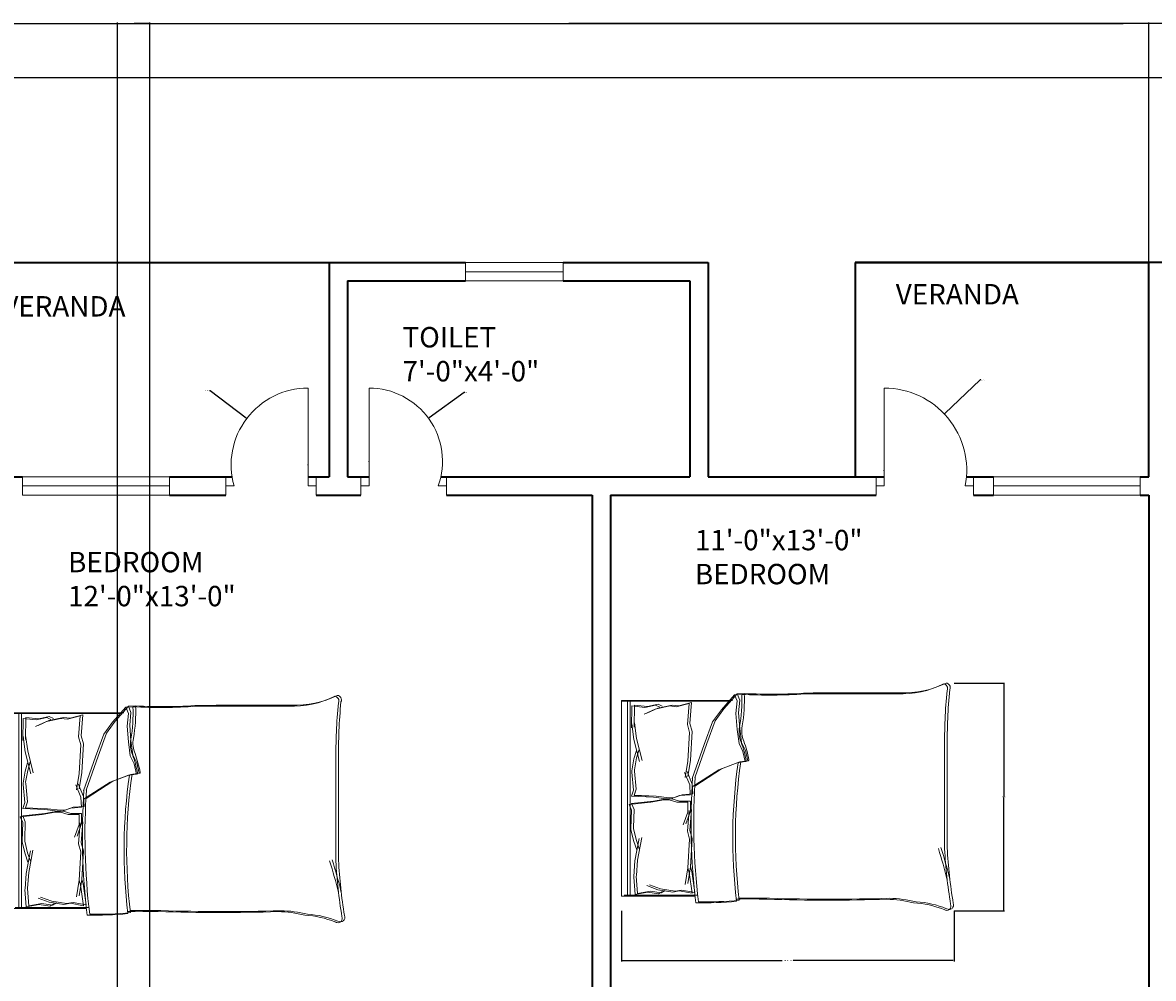
# Model space of a CAD drawing. Units: inches. Extents: x 2163 to 2982, y 1024 to 2288.
# Tile 18 of 22: x 2306 to 2583, y 2054 to 2288. Entities that reach past the tile are written whole.
import ezdxf

# ---------------------------------------------------------------- set-up
doc = ezdxf.new("R2010")
doc.units = ezdxf.units.IN
for name, color, linetype, lineweight in [('A-ANNO-DIMS', 2, 'Continuous', 18), ('A-ANNO-TTLB', 7, 'Continuous', 25), ('A-AREA-IDEN', 7, 'Continuous', 18), ('A-DOOR', 11, 'Continuous', 18), ('A-FURN', 8, 'Continuous', 13), ('A-GLAZ', 161, 'Continuous', 18), ('A-WALL', 7, 'Continuous', 35)]:
    doc.layers.add(name, color=color, linetype=linetype, lineweight=lineweight)
doc.styles.get("Standard").update_dxf_attribs({"font": 'arial.ttf'})
doc.dimstyles.get("Standard").update_dxf_attribs({"dimtxt": 0.18, "dimasz": 0.18, "dimexe": 0.18, "dimexo": 0.0625, "dimgap": 0.09, "dimtad": 0, "dimtih": 1, "dimtoh": 1, "dimdec": 4, "dimzin": 0, "dimdsep": 46, "dimtxsty": 'Standard', "dimcen": 0.09, "dimadec": 0, "dimazin": 0, "dimtfac": 1, "dimtdec": 4, "dimtofl": 0, "dimtmove": 0, "dimatfit": 3, "dimfxl": 1, "dimtolj": 1, "dimtzin": 0, "dimarcsym": 0})

# ---------------------------------------------------------------- blocks, each defined once
blk = doc.blocks.new('BED-DOUBLE')
for p, q in [((27.75, 52.87), (24.5, 49.16)), ((27.75, 52.87), (24.5, 49.16)), ((28.38, 53.1), (25.13, 49.39)), ((28.38, 53.1), (25.13, 49.39)), ((29.49, 52.95), (27.75, 52.87, 3.87)), ((29.49, 52.95), (27.75, 52.87, 3.87)), ((28.36, 51.33), (27.75, 52.87)), ((28.36, 51.33), (27.75, 52.87)), ((30.13, 53.18), (28.38, 53.1, 3.87)), ((29, 51.56), (28.38, 53.1)), ((30.13, 53.18), (28.38, 53.1, 3.87)), ((29, 51.56), (28.38, 53.1)), ((0, 51.49), (0.64, 51.49)), ((0, 3.47), (0, 51.49)), ((0, 51.27), (26.61, 51.27)), ((0, 51.27), (26.61, 51.27)), ((0.64, 51.49), (27.25, 51.49)), ((0.64, 51.49), (27.25, 51.49)), ((1.53, 3.48), (1.53, 51.27)), ((1.53, 3.47), (1.53, 51.27)), ((2.17, 3.7), (2.17, 51.49)), ((2.17, 3.7), (2.17, 51.49)), ((2.56, 50.11), (2.46, 44.71)), ((2.56, 50.11), (2.46, 44.71)), ((2.56, 50.11), (5.77, 49.73)), ((2.56, 50.11), (5.77, 49.73)), ((3.2, 50.34), (3.1, 44.94)), ((3.2, 50.34), (3.1, 44.94)), ((3.2, 50.34), (6.41, 49.96)), ((3.2, 50.34), (6.41, 49.96)), ((5.77, 49.73), (8.34, 50.33)), ((5.77, 49.73), (8.34, 50.33)), ((6.41, 49.96), (8.98, 50.56)), ((6.41, 49.96), (8.98, 50.56)), ((11.83, 50.11), (8.26, 49.31)), ((11.83, 50.11), (8.26, 49.31)), ((8.34, 50.33), (9.38, 49.81)), ((8.34, 50.33), (9.38, 49.81)), ((12.47, 50.34), (8.9, 49.54)), ((12.47, 50.34), (8.9, 49.54)), ((8.98, 50.56), (10.02, 50.04)), ((8.98, 50.56), (10.02, 50.04)), ((13.43, 49.92), (11.83, 50.11)), ((13.43, 49.92), (11.83, 50.11)), ((14.07, 50.15), (12.47, 50.34)), ((14.07, 50.15), (12.47, 50.34)), ((16.57, 50.7), (13.43, 49.92)), ((16.57, 50.7), (13.43, 49.92)), ((17.21, 50.93), (14.07, 50.15)), ((17.21, 50.93), (14.07, 50.15)), ((16.17, 45.57), (16.57, 50.7)), ((16.17, 45.57), (16.57, 50.7)), ((16.81, 45.79), (17.21, 50.93)), ((16.81, 45.79), (17.21, 50.93)), ((28.06, 48.23), (28.36, 51.33)), ((28.06, 48.23), (28.36, 51.33)), ((28.69, 48.46), (29, 51.56)), ((28.69, 48.46), (29, 51.56)), ((8.26, 49.31), (5.58, 48.13)), ((8.26, 49.31), (5.58, 48.13)), ((8.9, 49.54), (6.22, 48.36)), ((8.9, 49.54), (6.22, 48.36)), ((24.5, 49.16), (22.33, 46.22)), ((24.5, 49.16), (22.33, 46.22)), ((25.13, 49.39), (22.97, 46.45)), ((25.13, 49.39), (22.97, 46.45)), ((28.36, 44.36), (28.06, 48.23)), ((28.36, 44.36), (28.06, 48.23)), ((29, 44.59), (28.69, 48.46)), ((29, 44.59), (28.69, 48.46)), ((2.46, 44.71), (2.54, 45.71)), ((2.46, 44.71), (2.54, 45.71)), ((2.54, 45.71), (3.07, 41.91)), ((2.54, 45.71), (3.07, 41.91)), ((3.1, 44.94), (3.18, 45.94)), ((3.1, 44.94), (3.18, 45.94)), ((3.18, 45.94), (3.71, 42.14)), ((3.18, 45.94), (3.71, 42.14)), ((16.73, 43.61), (16.17, 45.57)), ((16.73, 43.61), (16.17, 45.57)), ((17.37, 43.83), (16.81, 45.79)), ((17.37, 43.83), (16.81, 45.79)), ((22.33, 46.22), (20.32, 40.64)), ((22.33, 46.22), (20.32, 40.64)), ((22.97, 46.45), (20.96, 40.87)), ((22.97, 46.45), (20.96, 40.87)), ((28.83, 40.95), (28.36, 44.36)), ((29.47, 41.18), (29, 44.59)), ((29.47, 41.18), (29, 44.59)), ((3.07, 41.91), (4.42, 36.49)), ((3.07, 41.91), (4.42, 36.49)), ((3.71, 42.14), (5.06, 36.72)), ((3.71, 42.14), (5.06, 36.72)), ((16.29, 36.6), (16.73, 43.61)), ((16.29, 36.6), (16.73, 43.61)), ((16.93, 36.82), (17.37, 43.83)), ((16.93, 36.82), (17.37, 43.83)), ((28.83, 40.95), (28.36, 44.36)), ((3.67, 39.2), (3.08, 37.14)), ((3.67, 39.2), (3.08, 37.13)), ((4.31, 39.43), (3.72, 37.36)), ((4.31, 39.43), (3.72, 37.36)), ((20.32, 40.64), (17.38, 32.31)), ((20.32, 40.64), (17.38, 32.31)), ((20.96, 40.87), (18.02, 32.53)), ((20.96, 40.87), (18.02, 32.53)), ((29.76, 38.94), (28.83, 40.95)), ((29.76, 38.94), (28.83, 40.95)), ((30.4, 39.17), (29.47, 41.18)), ((30.4, 39.17), (29.47, 41.18)), ((30.38, 36.46), (29.76, 38.94)), ((30.38, 36.46), (29.76, 38.94)), ((31.02, 36.69), (30.4, 39.17)), ((31.02, 36.69), (30.4, 39.17)), ((79.24, 15.06), (79.24, 39.68)), ((79.24, 15.06), (79.24, 39.68)), ((79.88, 15.29), (79.88, 39.91)), ((79.88, 15.29), (79.88, 39.91)), ((3.08, 37.14), (2.54, 34.2)), ((3.08, 37.13), (2.54, 34.2)), ((3.72, 37.36), (3.18, 34.43)), ((3.72, 37.36), (3.18, 34.43)), ((15.63, 32.56), (16.29, 36.6)), ((15.63, 32.56), (16.29, 36.6)), ((16.27, 32.79), (16.93, 36.82)), ((16.27, 32.79), (16.93, 36.82)), ((23.88, 34.45), (28.36, 36.15)), ((23.88, 34.45), (28.36, 36.15)), ((24.52, 34.68), (29, 36.38)), ((24.52, 34.68), (29, 36.38)), ((28.36, 36.15), (30.38, 36.46)), ((28.36, 36.15), (30.38, 36.46)), ((29, 36.38), (31.02, 36.69)), ((29, 36.38), (31.02, 36.69)), ((2.54, 34.2), (2.56, 33.88)), ((2.54, 34.2), (2.56, 33.88)), ((2.56, 33.88), (2.98, 29.46)), ((2.56, 33.88), (2.98, 29.46)), ((3.18, 34.43), (3.2, 34.11)), ((3.18, 34.43), (3.2, 34.11)), ((3.2, 34.11), (3.62, 29.68)), ((3.2, 34.11), (3.62, 29.68)), ((16.74, 30.75), (15.45, 33.82)), ((16.74, 30.75), (15.45, 33.82)), ((17.38, 30.98), (16.09, 34.05)), ((17.38, 30.98), (16.09, 34.05)), ((17.38, 30.26), (23.88, 34.45)), ((17.38, 30.26), (23.88, 34.45)), ((18.02, 30.49), (24.52, 34.68)), ((18.02, 30.49), (24.52, 34.68)), ((16.89, 28.3), (16.74, 30.75)), ((16.89, 28.3), (16.74, 30.75)), ((17.53, 28.53), (17.38, 30.98)), ((17.53, 28.53), (17.38, 30.98)), ((2.98, 29.46), (2.49, 27.98)), ((2.98, 29.46), (2.49, 27.98)), ((2.49, 27.98), (7.87, 27.73)), ((2.49, 27.98), (7.87, 27.73)), ((3.62, 29.68), (3.13, 28.21)), ((3.62, 29.68), (3.13, 28.2)), ((3.13, 28.21), (8.51, 27.96)), ((3.13, 28.2), (8.51, 27.96)), ((7.87, 27.73), (11.08, 27.35)), ((7.87, 27.73), (11.08, 27.35)), ((8.51, 27.96), (11.72, 27.58)), ((8.51, 27.96), (11.72, 27.58)), ((12.38, 27.44), (14.22, 28.13)), ((12.38, 27.44), (14.22, 28.13)), ((13.02, 27.66), (14.86, 28.36)), ((13.02, 27.66), (14.86, 28.36)), ((14.22, 28.13), (16.89, 28.3)), ((14.22, 28.13), (16.89, 28.3)), ((14.86, 28.36), (17.53, 28.53)), ((14.86, 28.36), (17.53, 28.53)), ((1.87, 25.98), (7.22, 26.56)), ((1.87, 25.98), (7.22, 26.56)), ((2.45, 24.54), (1.87, 25.98)), ((2.45, 24.54), (1.87, 25.98)), ((2.51, 26.21), (7.86, 26.79)), ((2.51, 26.21), (7.86, 26.79)), ((3.09, 24.77), (2.51, 26.21)), ((3.09, 24.77), (2.51, 26.21)), ((7.22, 26.56), (10.4, 27.14)), ((7.22, 26.56), (10.4, 27.14)), ((7.86, 26.79), (11.04, 27.37)), ((7.86, 26.79), (11.04, 27.37)), ((10.4, 27.14), (11.7, 27.14)), ((10.4, 27.14), (11.7, 27.14)), ((11.04, 27.37), (12.34, 27.37)), ((11.04, 27.37), (12.34, 27.37)), ((11.08, 27.35), (12.38, 27.44)), ((11.08, 27.35), (12.38, 27.44)), ((11.7, 27.14), (13.58, 26.56)), ((11.7, 27.14), (13.58, 26.56)), ((11.72, 27.58), (13.02, 27.66)), ((11.72, 27.58), (13.02, 27.66)), ((12.34, 27.37), (14.22, 26.79)), ((12.34, 27.37), (14.22, 26.79)), ((13.58, 26.56), (16.26, 26.56)), ((13.58, 26.56), (16.26, 26.56)), ((14.22, 26.79), (16.9, 26.79)), ((14.22, 26.79), (16.9, 26.79)), ((16.26, 26.56), (16.26, 24.1)), ((16.26, 26.56), (16.26, 24.1)), ((16.9, 26.79), (16.9, 24.33)), ((16.9, 26.79), (16.9, 24.33)), ((2.3, 20.09), (2.45, 24.54)), ((2.3, 20.09), (2.45, 24.54)), ((2.94, 20.32), (3.09, 24.77)), ((2.94, 20.32), (3.09, 24.77)), ((16.26, 24.1), (15.17, 20.96)), ((16.26, 24.1), (15.17, 20.96)), ((16.9, 24.33), (15.81, 21.19)), ((16.9, 24.33), (15.81, 21.19)), ((16.17, 19.38), (16.57, 24.52)), ((16.17, 19.38), (16.57, 24.52)), ((16.81, 19.61), (17.21, 24.74)), ((16.81, 19.61), (17.21, 24.74)), ((2.3, 19.77), (2.3, 20.09)), ((2.3, 19.77), (2.3, 20.09)), ((3.03, 16.88), (2.3, 19.77)), ((3.03, 16.88), (2.3, 19.77)), ((2.94, 20), (2.94, 20.32)), ((2.94, 20), (2.94, 20.32)), ((3.67, 17.11), (2.94, 20)), ((3.67, 17.11), (2.94, 20)), ((17.37, 17.65), (16.81, 19.61)), ((17.37, 17.65), (16.81, 19.61)), ((3.75, 14.85), (3.03, 16.88)), ((3.75, 14.85), (3.03, 16.88)), ((3.32, 12.11), (4.33, 17.6)), ((3.32, 12.11), (4.33, 17.6)), ((4.39, 15.08), (3.67, 17.11)), ((4.39, 15.08), (3.67, 17.11)), ((3.96, 12.34), (4.97, 17.83)), ((3.96, 12.34), (4.97, 17.83)), ((16.73, 17.42), (16.17, 19.38)), ((16.73, 17.42), (16.17, 19.38)), ((16.29, 10.41), (16.73, 17.42)), ((16.29, 10.41), (16.73, 17.42)), ((16.93, 10.64), (17.37, 17.65)), ((16.93, 10.64), (17.37, 17.65)), ((3.03, 8.28), (3.32, 12.11)), ((3.03, 8.28), (3.32, 12.11)), ((3.67, 8.51), (3.96, 12.34)), ((3.67, 8.51), (3.96, 12.34)), ((3.65, 8.41), (3.67, 8.51)), ((3.65, 8.41), (3.67, 8.51)), ((3.98, 4.13), (3.65, 8.41)), ((3.98, 4.13), (3.65, 8.41)), ((15.63, 6.38), (16.29, 10.41)), ((15.63, 6.38), (16.29, 10.41)), ((16.27, 6.61), (16.93, 10.64)), ((16.27, 6.61), (16.93, 10.64)), ((16.29, 10.41), (16.62, 9.28)), ((16.29, 10.41), (16.62, 9.28)), ((16.62, 9.28), (17.34, 4.18)), ((16.62, 9.28), (17.34, 4.18)), ((16.93, 10.64), (17.26, 9.51)), ((16.93, 10.64), (17.26, 9.51)), ((17.26, 9.51), (17.98, 4.41)), ((17.26, 9.51), (17.98, 4.41)), ((3.01, 8.18), (3.03, 8.28)), ((3.01, 8.18), (3.03, 8.28)), ((3.34, 3.9), (3.01, 8.18)), ((3.34, 3.9), (3.01, 8.18)), ((8.95, 5.05), (6.21, 6.06)), ((8.95, 5.05), (6.21, 6.06)), ((9.59, 5.28), (6.85, 6.29)), ((9.59, 5.28), (6.85, 6.29)), ((18.11, 3.48), (0, 3.48)), ((18.11, 3.47), (0, 3.47)), ((18.75, 3.7), (0.64, 3.7)), ((18.75, 3.7), (0.64, 3.7)), ((3.32, 3.89), (6.5, 4.47)), ((3.32, 3.89), (6.5, 4.47)), ((3.96, 4.12), (7.14, 4.7)), ((3.96, 4.12), (7.14, 4.7)), ((6.5, 4.47), (9.1, 4.04)), ((6.5, 4.47), (9.1, 4.04)), ((7.14, 4.7), (9.74, 4.27)), ((7.14, 4.7), (9.74, 4.27)), ((12.57, 4.47), (8.95, 5.05)), ((12.57, 4.47), (8.95, 5.05)), ((9.1, 4.04), (10.11, 4.62)), ((9.1, 4.04), (10.11, 4.62)), ((13.21, 4.7), (9.59, 5.28)), ((13.21, 4.7), (9.59, 5.28)), ((9.74, 4.27), (10.75, 4.85)), ((9.74, 4.27), (10.75, 4.85)), ((14.16, 4.76), (12.57, 4.47)), ((14.16, 4.76), (12.57, 4.47)), ((14.8, 4.99), (13.21, 4.7)), ((14.8, 4.99), (13.21, 4.7)), ((17.34, 4.18), (14.16, 4.76)), ((17.34, 4.18), (14.16, 4.76)), ((17.98, 4.41), (14.8, 4.99)), ((17.98, 4.41), (14.8, 4.99))]:
    blk.add_line(p, q)
for centre, radius, start, end in [((68.67, 76.16), 23.07, 267.4714, 296.4681), ((68.67, 76.16), 23.07, 267.4714, 296.4681), ((69.31, 76.39), 23.07, 267.4714, 296.4681), ((69.31, 76.39), 23.07, 267.4714, 296.4681), ((78.87, 54.41), 1.1, 332.6588, 86.02), ((78.87, 54.41), 1.1, 332.6588, 86.02), ((79.51, 54.64), 1.1, 332.6588, 86.02), ((79.51, 54.64), 1.1, 332.6588, 86.02), ((-6.66, 51.33), 36.18, 349.8763, 2.5657), ((-6.66, 51.33), 36.18, 349.8763, 2.5657), ((36.31, 182.27), 129.5, 266.9791, 273.8365), ((36.31, 182.27), 129.5, 266.9791, 273.8365), ((-6.02, 51.56), 36.18, 349.8763, 2.5657), ((-6.02, 51.56), 36.18, 349.8763, 2.5657), ((36.95, 182.49), 129.5, 266.9791, 273.8365), ((36.95, 182.49), 129.5, 266.9791, 273.8365), ((67.82, -4508.74), 4561.86, 90.00217, 90.28689), ((67.82, -4508.74), 4561.86, 90.00217, 90.28689), ((68.46, -4508.52), 4561.86, 90.00217, 90.28689), ((68.46, -4508.52), 4561.86, 90.00217, 90.28689), ((212.28, 41.15), 133.04, 174.4998, 180.6351), ((212.28, 41.15), 133.04, 174.4998, 180.6351), ((212.92, 41.38), 133.04, 174.4998, 180.6351), ((212.92, 41.38), 133.04, 174.4998, 180.6351), ((35.07, 43.74), 6.22, 168.6608, 203.7384), ((35.07, 43.74), 6.22, 168.6608, 203.7384), ((35.71, 43.97), 6.22, 168.6608, 203.7384), ((35.71, 43.97), 6.22, 168.6608, 203.7384), ((1.48, 31.15), 29.65, 10.6617, 19.8806), ((1.48, 31.15), 29.65, 10.6617, 19.8806), ((2.12, 31.38), 29.65, 10.6617, 19.8806), ((2.12, 31.38), 29.65, 10.6617, 19.8806), ((156.32, 17.76), 129.02, 171.7845, 186.9006), ((156.32, 17.76), 129.02, 171.7845, 186.9006), ((156.96, 17.98), 129.02, 171.7845, 186.9006), ((156.96, 17.98), 129.02, 171.7845, 186.9006), ((30.44, 36.64), 0.185, 250.2464, 1.1377), ((30.44, 36.64), 0.185, 250.2464, 1.1377), ((31.08, 36.86), 0.185, 250.2464, 1.1377), ((31.08, 36.86), 0.185, 250.2464, 1.1377), ((182.05, 21.36), 164.97, 176.0865, 186.7821), ((182.05, 21.36), 164.97, 176.0865, 186.7821), ((182.69, 21.59), 164.97, 176.0865, 186.7821), ((182.69, 21.59), 164.97, 176.0865, 186.7821), ((-23.71, -17.22), 106.46, 13.3832, 17.7053), ((-23.71, -17.22), 106.46, 13.3832, 17.7053), ((-23.07, -16.99), 106.46, 13.3832, 17.7053), ((-23.07, -16.99), 106.46, 13.3832, 17.7053), ((200.84, 21.43), 121.76, 182.9958, 189.4091), ((200.84, 21.43), 121.76, 182.9958, 189.4091), ((201.48, 21.66), 121.76, 182.9958, 189.4091), ((201.48, 21.65), 121.76, 182.9958, 189.4091), ((31.17, -167.31), 170.11, 88.4762, 91.0082), ((31.17, -167.31), 170.11, 88.4762, 91.0082), ((31.81, -167.08), 170.11, 88.4762, 91.0082), ((31.81, -167.08), 170.11, 88.4762, 91.0082), ((51.25, 485.05), 482.31, 268.2277, 271.7185), ((51.25, 485.05), 482.31, 268.2277, 271.7185), ((65.15, -26.67), 29.63, 76.0648, 88.9113), ((65.15, -26.67), 29.63, 76.0648, 88.9113), ((20.1, 85.16), 83.31, 268.7218, 275.604), ((20.1, 85.16), 83.31, 268.7218, 275.604), ((20.74, 85.39), 83.31, 268.7218, 275.604), ((20.74, 85.39), 83.31, 268.7218, 275.604), ((50.61, 484.82), 482.31, 268.2277, 271.7185), ((50.61, 484.82), 482.31, 268.2277, 271.7185), ((64.51, -26.9), 29.63, 76.0648, 88.9113), ((64.51, -26.9), 29.63, 76.0648, 88.9113), ((70.28, -21.66), 23.56, 67.9751, 86.652), ((70.28, -21.66), 23.56, 67.9751, 86.652), ((70.91, -21.43), 23.56, 67.9751, 86.652), ((70.91, -21.43), 23.56, 67.9751, 86.652), ((79.72, 1.09), 1.09, 236.1736, 23.4781), ((79.72, 1.09), 1.09, 236.1736, 23.4781), ((80.36, 1.32), 1.09, 236.1736, 23.4781), ((80.36, 1.32), 1.09, 236.1736, 23.4781)]:
    blk.add_arc(centre, radius, start, end)
blk = doc.blocks.new('WIN-24')
for p, q in [((0, 24), (4.5, 24)), ((0, 24), (0, 0)), ((4.5, 24), (2.25, 24)), ((2.25, 24), (2.25, 0)), ((4.5, 24), (4.5, 0)), ((2.25, 0), (0, 0)), ((0, 0), (4.5, 0))]:
    blk.add_line(p, q)
blk = doc.blocks.new('WIN-36')
for p, q in [((2.25, 36), (0, 36)), ((0, 36), (4.5, 36)), ((0, 36), (0, 0)), ((2.25, 0), (2.25, 36)), ((4.5, 36), (4.5, 0)), ((0, 0), (4.5, 0)), ((4.5, 0), (2.25, 0))]:
    blk.add_line(p, q)
blk = doc.blocks.new('WIN-36-ALT')
for p, q in [((2.25, 36), (0, 36)), ((0, 36), (4.5, 36)), ((0, 36), (0, 0)), ((2.25, 0), (2.25, 36)), ((4.5, 36), (4.5, 0)), ((4.5, 0), (0, 0)), ((0, 0), (2.25, 0))]:
    blk.add_line(p, q)
blk = doc.blocks.new('*D9')
at = {"layer": 'A-ANNO-DIMS', "color": 0, "lineweight": -2, "transparency": 16777216}
for p, q in [((2453.03, 2070.32), (2453.03, 2057.97)), ((2534.58, 2070.32), (2534.58, 2057.97)), ((2453.21, 2058.15), (2492.44, 2058.15)), ((2534.4, 2058.15), (2495.17, 2058.15))]:
    blk.add_line(p, q, dxfattribs=at)
at = {"layer": 'A-ANNO-DIMS', "color": 0, "transparency": 16777216}
for points in [[(2453.21, 2058.18), (2453.21, 2058.12), (2453.03, 2058.15)], [(2534.4, 2058.18), (2534.4, 2058.12), (2534.58, 2058.15)]]:
    blk.add_solid(points, dxfattribs=at)
at = {"layer": 'Defpoints', "color": 0, "transparency": 16777216}
for p in [(2453.03, 2070.38), (2534.58, 2070.38), (2534.58, 2058.15)]:
    blk.add_point(p, dxfattribs=at)
at = {"layer": 'A-ANNO-DIMS', "color": 0, "transparency": 16777216, "insert": (2493.8, 2058.15), "char_height": 0.18, "attachment_point": 5}
blk.add_mtext('\\A1;DOUBLE BED 82 TYP.', dxfattribs=at)
blk = doc.blocks.new('*D10')
at = {"layer": 'A-ANNO-DIMS', "color": 0, "lineweight": -2, "transparency": 16777216}
for p, q in [((2534.64, 2126.21), (2546.99, 2126.21)), ((2546.81, 2126.03), (2546.81, 2098.48)), ((2546.81, 2070.56), (2546.81, 2098.11)), ((2534.64, 2070.38), (2546.99, 2070.38))]:
    blk.add_line(p, q, dxfattribs=at)
at = {"layer": 'A-ANNO-DIMS', "color": 0, "transparency": 16777216}
for points in [[(2546.78, 2126.03), (2546.84, 2126.03), (2546.81, 2126.21)], [(2546.78, 2070.56), (2546.84, 2070.56), (2546.81, 2070.38)]]:
    blk.add_solid(points, dxfattribs=at)
at = {"layer": 'Defpoints', "color": 0, "transparency": 16777216}
for p in [(2534.58, 2126.21), (2546.81, 2126.21), (2534.58, 2070.38)]:
    blk.add_point(p, dxfattribs=at)
at = {"layer": 'A-ANNO-DIMS', "color": 0, "transparency": 16777216, "insert": (2546.81, 2098.3), "char_height": 0.18, "attachment_point": 5}
blk.add_mtext('\\A1;56 TYP.', dxfattribs=at)
blk = doc.blocks.new('*D28')
at = {"layer": 'A-ANNO-DIMS', "color": 0, "lineweight": -2, "transparency": 16777216}
for p, q in [((2297.34, 2229.33), (2297.34, 2288.1)), ((2297.52, 2287.92), (2439.55, 2287.92)), ((2582.16, 2287.92), (2440.13, 2287.92)), ((2582.34, 2229.33), (2582.34, 2288.1))]:
    blk.add_line(p, q, dxfattribs=at)
at = {"layer": 'A-ANNO-DIMS', "color": 0, "transparency": 16777216}
for points in [[(2297.52, 2287.95), (2297.52, 2287.89), (2297.34, 2287.92)], [(2582.16, 2287.95), (2582.16, 2287.89), (2582.34, 2287.92)]]:
    blk.add_solid(points, dxfattribs=at)
at = {"layer": 'Defpoints', "color": 0, "transparency": 16777216}
for p in [(2582.34, 2287.92), (2297.34, 2229.27), (2582.34, 2229.27)]:
    blk.add_point(p, dxfattribs=at)
at = {"layer": 'A-ANNO-DIMS', "color": 0, "transparency": 16777216, "insert": (2439.84, 2287.92), "char_height": 0.18, "attachment_point": 5}
blk.add_mtext('\\A1;285', dxfattribs=at)
blk = doc.blocks.new('*D29')
at = {"layer": 'A-ANNO-DIMS', "color": 0, "lineweight": -2, "transparency": 16777216}
for p, q in [((2285.34, 1738.83), (2285.34, 2288.1)), ((2285.52, 2287.92), (2576.05, 2287.92)), ((2867.16, 2287.92), (2576.63, 2287.92)), ((2867.34, 2229.33), (2867.34, 2288.1))]:
    blk.add_line(p, q, dxfattribs=at)
at = {"layer": 'A-ANNO-DIMS', "color": 0, "transparency": 16777216}
for points in [[(2285.52, 2287.95), (2285.52, 2287.89), (2285.34, 2287.92)], [(2867.16, 2287.95), (2867.16, 2287.89), (2867.34, 2287.92)]]:
    blk.add_solid(points, dxfattribs=at)
at = {"layer": 'Defpoints', "color": 0, "transparency": 16777216}
for p in [(2867.34, 2287.92), (2867.34, 2229.27), (2285.34, 1738.77)]:
    blk.add_point(p, dxfattribs=at)
at = {"layer": 'A-ANNO-DIMS', "color": 0, "transparency": 16777216, "insert": (2576.34, 2287.92), "char_height": 0.18, "attachment_point": 5}
blk.add_mtext('\\A1;582', dxfattribs=at)
blk = doc.blocks.new('*D38')
at = {"layer": 'A-ANNO-DIMS', "color": 0, "lineweight": -2, "transparency": 16777216}
for p, q in [((2329.44, 1734.33), (2329.44, 2288.1)), ((2329.62, 2287.92), (2333.29, 2287.92)), ((2337.26, 2287.92), (2333.59, 2287.92)), ((2337.44, 1734.33), (2337.44, 2288.1))]:
    blk.add_line(p, q, dxfattribs=at)
at = {"layer": 'A-ANNO-DIMS', "color": 0, "transparency": 16777216}
for points in [[(2329.62, 2287.95), (2329.62, 2287.89), (2329.44, 2287.92)], [(2337.26, 2287.95), (2337.26, 2287.89), (2337.44, 2287.92)]]:
    blk.add_solid(points, dxfattribs=at)
at = {"layer": 'Defpoints', "color": 0, "transparency": 16777216}
for p in [(2337.44, 2287.92), (2329.44, 1734.27), (2337.44, 1734.27)]:
    blk.add_point(p, dxfattribs=at)
at = {"layer": 'A-ANNO-DIMS', "color": 0, "transparency": 16777216, "insert": (2333.44, 2287.92), "char_height": 0.18, "attachment_point": 5}
blk.add_mtext('\\A1;8', dxfattribs=at)
blk = doc.blocks.new('*D57')
at = {"layer": 'A-ANNO-DIMS', "color": 0, "lineweight": -2, "transparency": 16777216}
for p, q in [((2352.01, 2197.95), (2352.19, 2197.95)), ((2352.19, 2197.95), (2361.05, 2191.2)), ((2376.1, 2179.67), (2376.28, 2179.67)), ((2376.19, 2179.58), (2376.19, 2179.76))]:
    blk.add_line(p, q, dxfattribs=at)
at = {"layer": 'A-ANNO-DIMS', "color": 0, "transparency": 16777216}
blk.add_solid([(2361.07, 2191.22), (2361.03, 2191.18), (2361.19, 2191.09)], dxfattribs=at)
at = {"layer": 'Defpoints', "color": 0, "transparency": 16777216}
for p in [(2361.19, 2191.09), (2376.19, 2179.67)]:
    blk.add_point(p, dxfattribs=at)
at = {"layer": 'A-ANNO-DIMS', "color": 0, "transparency": 16777216, "insert": (2351.47, 2197.95), "char_height": 0.18, "attachment_point": 5}
blk.add_mtext('\\A1;R18.854', dxfattribs=at)
blk = doc.blocks.new('*D58')
at = {"layer": 'A-ANNO-DIMS', "color": 0, "lineweight": -2, "transparency": 16777216}
for p, q in [((2414.48, 2197.42), (2405.88, 2191.19)), ((2414.66, 2197.42), (2414.48, 2197.42)), ((2391.07, 2180.52), (2391.25, 2180.52)), ((2391.16, 2180.43), (2391.16, 2180.61))]:
    blk.add_line(p, q, dxfattribs=at)
at = {"layer": 'A-ANNO-DIMS', "color": 0, "transparency": 16777216}
blk.add_solid([(2405.86, 2191.21), (2405.9, 2191.16), (2405.73, 2191.08)], dxfattribs=at)
at = {"layer": 'Defpoints', "color": 0, "transparency": 16777216}
for p in [(2405.73, 2191.08), (2391.16, 2180.52)]:
    blk.add_point(p, dxfattribs=at)
at = {"layer": 'A-ANNO-DIMS', "color": 0, "transparency": 16777216, "insert": (2414.96, 2197.42), "char_height": 0.18, "attachment_point": 5}
blk.add_mtext('\\A1;R18', dxfattribs=at)
blk = doc.blocks.new('*D59')
at = {"layer": 'A-ANNO-DIMS', "color": 0, "lineweight": -2, "transparency": 16777216}
for p, q in [((2541.01, 2200.5), (2532.31, 2192.3)), ((2541.19, 2200.5), (2541.01, 2200.5)), ((2517.38, 2178.3), (2517.56, 2178.3)), ((2517.47, 2178.21), (2517.47, 2178.39))]:
    blk.add_line(p, q, dxfattribs=at)
at = {"layer": 'A-ANNO-DIMS', "color": 0, "transparency": 16777216}
blk.add_solid([(2532.29, 2192.32), (2532.33, 2192.27), (2532.18, 2192.17)], dxfattribs=at)
at = {"layer": 'Defpoints', "color": 0, "transparency": 16777216}
for p in [(2532.18, 2192.17), (2517.47, 2178.3)]:
    blk.add_point(p, dxfattribs=at)
at = {"layer": 'A-ANNO-DIMS', "color": 0, "transparency": 16777216, "insert": (2541.67, 2200.5), "char_height": 0.18, "attachment_point": 5}
blk.add_mtext('\\A1;R20.22', dxfattribs=at)

msp = doc.modelspace()

# ---------------------------------------------------------------- linework, layer by layer
at = {"layer": 'A-ANNO-TTLB'}
msp.add_lwpolyline([(2162.6841, 2274.6054), (2982.469, 2274.6054), (2982.469, 1045.9691), (2162.6841, 1045.9691)], close=True, dxfattribs=at)
at = {"layer": 'A-DOOR'}
for p, q in [((2376.1895, 2174.5188), (2376.1895, 2198.5188)), ((2391.1617, 2174.5188), (2391.1617, 2198.5188)), ((2517.4715, 2174.5188), (2517.4715, 2198.5188)), ((2356.0519, 2176.7688), (2356.0519, 2172.2688)), ((2378.1895, 2176.7688), (2378.1895, 2172.2688)), ((2389.1617, 2176.7688), (2389.1617, 2172.2688)), ((2410.1301, 2176.7688), (2410.1301, 2172.2688)), ((2515.4715, 2176.7688), (2515.4715, 2172.2688)), ((2539.3372, 2176.7688), (2539.3372, 2172.2688)), ((2356.0519, 2172.2688), (2356.0519, 2174.5188)), ((2356.0519, 2174.5188), (2358.0519, 2174.5188)), ((2378.1895, 2174.5188), (2376.1895, 2174.5188)), ((2378.1895, 2172.2688), (2378.1895, 2174.5188)), ((2389.1617, 2172.2688), (2389.1617, 2174.5188)), ((2389.1617, 2174.5188), (2391.1617, 2174.5188)), ((2410.1301, 2174.5188), (2408.1301, 2174.5188)), ((2410.1301, 2172.2688), (2410.1301, 2174.5188)), ((2515.4715, 2172.2688), (2515.4715, 2174.5188)), ((2515.4715, 2174.5188), (2517.4715, 2174.5188)), ((2539.3372, 2174.5188), (2537.3372, 2174.5188)), ((2539.3372, 2172.2688), (2539.3372, 2174.5188))]:
    msp.add_line(p, q, dxfattribs=at)
for centre, radius, start, end in [((2376.1895, 2179.6653), 18.8535, 90, 195.841076), ((2391.1617, 2180.5204), 17.9985, 340.521857, 90), ((2517.4715, 2178.2971), 20.2218, 349.231572, 90)]:
    msp.add_arc(centre, radius, start, end, dxfattribs=at)
at = {"layer": 'A-WALL'}
for p, q in [((2297.3389, 2229.2688), (2414.7613, 2229.2688)), ((2381.3389, 2229.2688), (2381.3389, 2176.7688)), ((2438.7613, 2229.2688), (2474.3389, 2229.2688)), ((2474.3389, 2229.2688), (2474.3389, 2176.7688)), ((2586.8389, 2229.2688), (2510.3389, 2229.2688)), ((2510.3389, 2229.2688), (2510.3389, 2176.7688)), ((2510.3389, 2229.2688), (2582.3389, 2229.2688)), ((2582.3389, 2176.7688), (2582.3389, 2229.2688)), ((2385.8389, 2224.7688), (2385.8389, 2176.7688)), ((2385.8389, 2224.7688), (2414.7613, 2224.7688)), ((2438.7613, 2224.7688), (2469.8389, 2224.7688)), ((2469.8389, 2224.7688), (2469.8389, 2176.7688)), ((2297.3389, 2176.7688), (2306.2073, 2176.7688)), ((2342.2073, 2176.7688), (2357.5597, 2176.7688)), ((2376.1895, 2176.7688), (2381.3389, 2176.7688)), ((2385.8389, 2176.7688), (2391.1617, 2176.7688)), ((2408.7649, 2176.7688), (2469.8389, 2176.7688)), ((2474.3389, 2176.7688), (2517.4715, 2176.7688)), ((2537.6355, 2176.7688), (2544.2576, 2176.7688)), ((2580.2576, 2176.7688), (2582.3389, 2176.7688)), ((2342.2073, 2172.2688), (2356.0519, 2172.2688)), ((2378.1895, 2172.2688), (2389.1617, 2172.2688)), ((2410.1301, 2172.2688), (2445.8389, 2172.2688)), ((2445.8389, 2172.2688), (2445.8389, 2016.2688)), ((2450.3389, 2172.2688), (2450.3389, 2016.2688)), ((2450.3389, 2172.2688), (2515.4715, 2172.2688)), ((2539.3372, 2172.2688), (2544.2576, 2172.2688)), ((2580.2576, 2172.2688), (2582.3389, 2172.2688)), ((2582.3389, 2172.2688), (2582.3389, 2016.2688))]:
    msp.add_line(p, q, dxfattribs=at)

# ---------------------------------------------------------------- block references
at = {"layer": 'A-FURN'}
for p in [(2453.0307, 2070.4701), (2303.774, 2067.438)]:
    msp.add_blockref('BED-DOUBLE', p, dxfattribs=at)
at = {"layer": 'A-GLAZ', "extrusion": (0, 0, -1), "zscale": -1, "rotation": 90}
msp.add_blockref('WIN-24', (-2414.7618, 2224.7689), dxfattribs=at)
at = {"layer": 'A-GLAZ', "rotation": 270}
for name, p in [('WIN-36-ALT', (2306.2078, 2176.7688)), ('WIN-36', (2544.2571, 2176.7688))]:
    msp.add_blockref(name, p, dxfattribs=at)

# ---------------------------------------------------------------- texts
at = {"layer": 'A-AREA-IDEN', "char_height": 5, "attachment_point": 1}
for s, width, insert in [('VERANDA', 24.43538, (2520.2979, 2224.0195)), ('VERANDA', 48.491843, (2301.2277, 2221.0494)), ('TOILET\\P7\'-0"x4\'-0"', 49.792106, (2399.3587, 2213.4804)), ('11\'-0"x13\'-0"\\PBEDROOM', 91.202676, (2471.0444, 2163.7456)), ('BEDROOM\\P12\'-0"x13\'-0"', 87.646653, (2317.3546, 2158.3525))]:
    msp.add_mtext_dynamic_manual_height_columns(s, width=width, gutter_width=12.5, heights=[0], dxfattribs=dict(at, insert=insert))

# ---------------------------------------------------------------- dimensions: what is measured, and where the dimension line sits
at = {"layer": 'A-ANNO-DIMS'}
for base, p1, p2, picture, middle in [((2867.3389, 2287.9188), (2285.3389, 1738.7688), (2867.3389, 2229.2688), '*D29', (2576.3389, 2287.9188)), ((2582.3389, 2287.9188), (2297.3389, 2229.2688), (2582.3389, 2229.2688), '*D28', (2439.8389, 2287.9188)), ((2337.4434, 2287.9188), (2329.4434, 1734.2688), (2337.4434, 1734.2688), '*D38', (2333.4434, 2287.9188))]:
    dim = msp.add_linear_dim(base=base, p1=p1, p2=p2, dimstyle='Standard', override={"dimdec": 0, "dimlfac": 1, "dimrnd": 0, "dimzin": 0, "dimdsep": 46, "dimlunit": 2}, dxfattribs=at)
    dim.commit()
    dim.dimension.update_dxf_attribs({"geometry": picture, "text_midpoint": middle})
for center, mpoint, override, picture, middle in [((2517.4715, 2178.2971), (2532.1823, 2192.172), {"dimdec": 2, "dimlfac": 1, "dimrnd": 0, "dimzin": 0, "dimdsep": 46, "dimlunit": 2}, '*D59', (2541.6677, 2200.4969)), ((2376.1895, 2179.6653), (2361.1927, 2191.0913), {"dimdec": 3, "dimlfac": 1, "dimrnd": 0, "dimzin": 0, "dimdsep": 46, "dimlunit": 2}, '*D57', (2351.4652, 2197.9469)), ((2391.1617, 2180.5204), (2405.7348, 2191.083), {"dimdec": 0, "dimlfac": 1, "dimrnd": 0, "dimzin": 0, "dimdsep": 46, "dimlunit": 2}, '*D58', (2414.9639, 2197.4206))]:
    dim = msp.add_radius_dim(center=center, mpoint=mpoint, dimstyle='Standard', override=override, dxfattribs=at)
    dim.commit()
    dim.dimension.update_dxf_attribs({"geometry": picture, "text_midpoint": middle, "dimtype": 164})
dim = msp.add_linear_dim(base=(2546.8113, 2126.208), p1=(2534.5791, 2070.3835), p2=(2534.5791, 2126.208), angle=90, text='<> TYP.', dimstyle='Standard', override={"dimdec": 0, "dimlfac": 1, "dimrnd": 0, "dimzin": 0, "dimdsep": 46, "dimlunit": 2}, dxfattribs=at)
dim.commit()
dim.dimension.update_dxf_attribs({"geometry": '*D10', "text_midpoint": (2546.8113, 2098.2958)})
dim = msp.add_linear_dim(base=(2534.5791, 2058.1512), p1=(2453.0304, 2070.3835), p2=(2534.5791, 2070.3835), text='DOUBLE BED <> TYP.', dimstyle='Standard', override={"dimdec": 0, "dimlfac": 1, "dimrnd": 0, "dimzin": 0, "dimdsep": 46, "dimlunit": 2}, dxfattribs=at)
dim.commit()
dim.dimension.update_dxf_attribs({"geometry": '*D9', "text_midpoint": (2493.8047, 2058.1512)})

doc.saveas('drawing.dxf')
